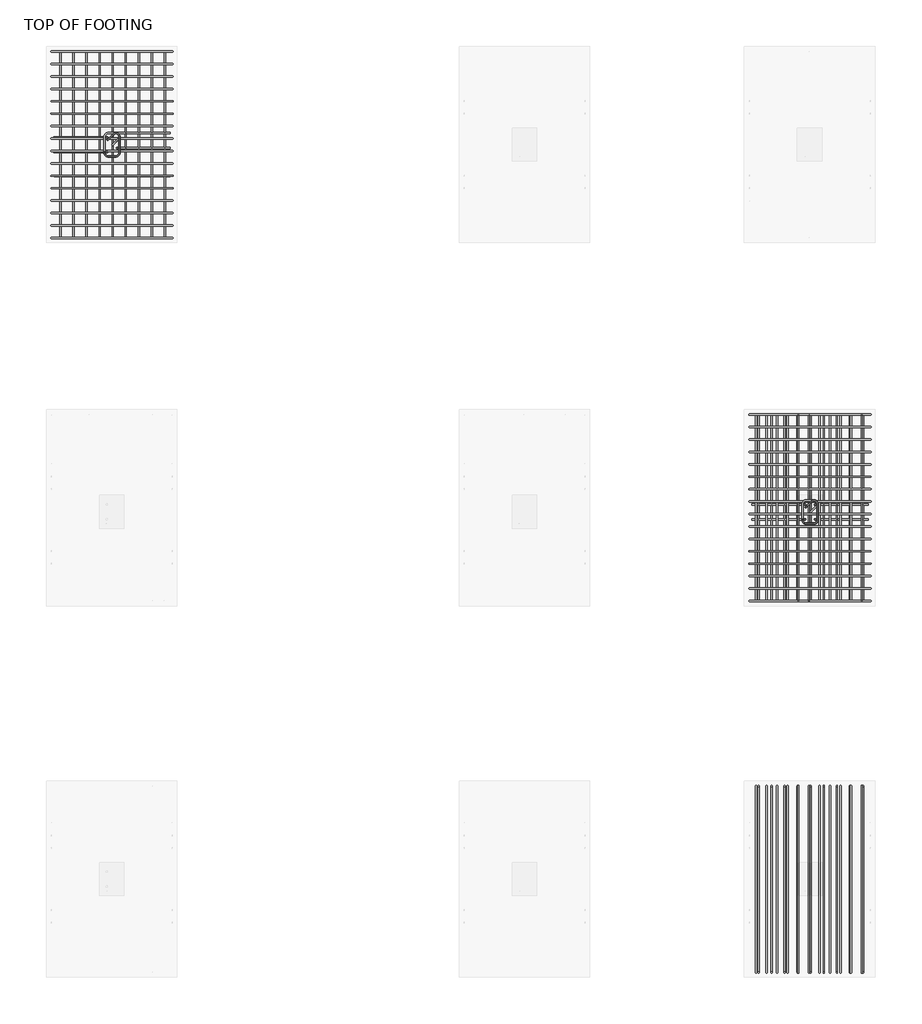
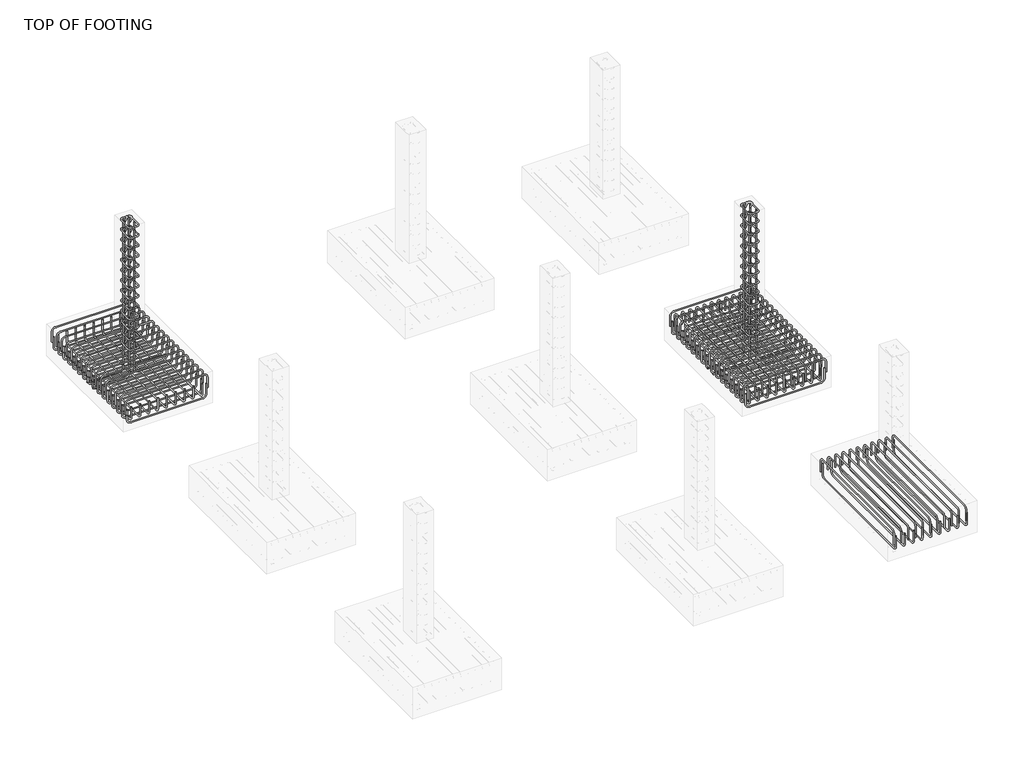
# One storey, part 7 of 8: 15 reinforcing bars.
"""IFC4 building model written with IfcOpenShell, lengths in millimetres."""

from ifc_helpers import new_model, si_unit, point, frame, origin, place, context, project, spatial, polyline, circle_curve, trimmed, segment, composite_curve, source, transform, mapped, element, save
from ifc_brep_helpers import swept_disk

model = new_model("IFC4")

# Units and contexts
model_context = context("Model", 3, world=origin())
ifc_project = project(units=[si_unit("LENGTHUNIT", "METRE", prefix="MILLI")], contexts=[model_context])

# Site, building, storey
site = spatial("IfcSite", under=ifc_project)
building = spatial("IfcBuilding", under=site)
storey = spatial("IfcBuildingStorey", under=building, Name="TOP OF FOOTING", Elevation=-1828.8)

# Reinforcing bars
placement = place(None, origin())
reinforcing_bar_shape = source(origin(), model_context, "Body", "SolidModel", [
    swept_disk(composite_curve([segment(polyline([(3061.4817577, 8966.4007933, -46.35), (3117.2253207, 9022.1443562, -46.35)]), True, "CONTINUOUS"), segment(trimmed(circle_curve(frame((3139.3931183, 8999.9765586, -46.35), z_axis=(0.0, 0.0, -1.0), x_axis=(-22.167797600000085, 22.167797600000995, 0.0)), 31.35), [point((3117.2253207, 9022.1443562, -46.35))], [point((3170.7431183, 8999.9765586, -46.35))], True, "CARTESIAN"), True, "CONTINUOUS"), segment(polyline([(3170.7431183, 8999.9765586, -46.35), (3170.7431183, 8850.5765586, -46.35)]), True, "CONTINUOUS"), segment(trimmed(circle_curve(frame((3139.3931183, 8850.5765586, -46.35), z_axis=(0.0, 0.0, -1.0), x_axis=(31.34999999999991, 0.0, 0.0)), 31.35), [point((3170.7431183, 8850.5765586, -46.35))], [point((3139.3931183, 8819.2265586, -46.35))], True, "CARTESIAN"), True, "CONTINUOUS"), segment(polyline([(3139.3931183, 8819.2265586, -46.35), (3066.1931183, 8819.2265586, -46.35)]), True, "CONTINUOUS"), segment(trimmed(circle_curve(frame((3066.1931183, 8850.5205096, -44.4761991), z_axis=(0.0, 0.05977036468717588, -0.9982121535551258), x_axis=(0.0, -31.29395100000147, -1.873800899999999)), 31.35), [point((3066.1931183, 8819.2265586, -46.35))], [point((3034.8431183, 8850.5205096, -44.4761991))], True, "CARTESIAN"), True, "CONTINUOUS"), segment(polyline([(3034.8431183, 8850.5205096, -44.4761991), (3034.8431183, 9000.0326076, -35.5238009)]), True, "CONTINUOUS"), segment(trimmed(circle_curve(frame((3066.1931183, 9000.0326076, -35.5238009), z_axis=(0.0, 0.05977036468717588, -0.9982121535551258), x_axis=(-31.350000000000364, 0.0, 0.0)), 31.35), [point((3034.8431183, 9000.0326076, -35.5238009))], [point((3066.1931183, 9031.3265586, -33.65))], True, "CARTESIAN"), True, "CONTINUOUS"), segment(polyline([(3066.1931183, 9031.3265586, -33.65), (3139.3931183, 9031.3265586, -33.65)]), True, "CONTINUOUS"), segment(trimmed(circle_curve(frame((3139.3931183, 8999.9765586, -33.65), z_axis=(0.0, 0.0, -1.0), x_axis=(0.0, 31.350000000000364, 0.0)), 31.35), [point((3139.3931183, 9031.3265586, -33.65))], [point((3161.5609159, 8977.808761, -33.65))], True, "CARTESIAN"), True, "CONTINUOUS"), segment(polyline([(3161.5609159, 8977.808761, -33.65), (3105.8173529, 8922.0651981, -33.65)]), True, "CONTINUOUS")], self_intersect=False), 6.35),
])
element("IfcReinforcingBar", 1, at=placement, inside=storey, context=model_context, shape_type="MappedRepresentation", body=[
    mapped(reinforcing_bar_shape, transform((0.0, 0.0, 0.0), x_axis=(1.0, 0.0, 0.0), y_axis=(0.0, 1.0, 0.0), z_axis=(0.0, 0.0, 1.0))),
    mapped(reinforcing_bar_shape, transform((0.0, 0.0, -144.675), x_axis=(1.0, 0.0, 0.0), y_axis=(0.0, 1.0, 0.0), z_axis=(0.0, 0.0, 1.0))),
    mapped(reinforcing_bar_shape, transform((0.0, 0.0, -289.35), x_axis=(1.0, 0.0, 0.0), y_axis=(0.0, 1.0, 0.0), z_axis=(0.0, 0.0, 1.0))),
    mapped(reinforcing_bar_shape, transform((0.0, 0.0, -434.025), x_axis=(1.0, 0.0, 0.0), y_axis=(0.0, 1.0, 0.0), z_axis=(0.0, 0.0, 1.0))),
    mapped(reinforcing_bar_shape, transform((0.0, 0.0, -578.7), x_axis=(1.0, 0.0, 0.0), y_axis=(0.0, 1.0, 0.0), z_axis=(0.0, 0.0, 1.0))),
    mapped(reinforcing_bar_shape, transform((0.0, 0.0, -723.375), x_axis=(1.0, 0.0, 0.0), y_axis=(0.0, 1.0, 0.0), z_axis=(0.0, 0.0, 1.0))),
    mapped(reinforcing_bar_shape, transform((0.0, 0.0, -868.05), x_axis=(1.0, 0.0, 0.0), y_axis=(0.0, 1.0, 0.0), z_axis=(0.0, 0.0, 1.0))),
    mapped(reinforcing_bar_shape, transform((0.0, 0.0, -1012.725), x_axis=(1.0, 0.0, 0.0), y_axis=(0.0, 1.0, 0.0), z_axis=(0.0, 0.0, 1.0))),
    mapped(reinforcing_bar_shape, transform((0.0, 0.0, -1157.4), x_axis=(1.0, 0.0, 0.0), y_axis=(0.0, 1.0, 0.0), z_axis=(0.0, 0.0, 1.0))),
    mapped(reinforcing_bar_shape, transform((0.0, 0.0, -1302.075), x_axis=(1.0, 0.0, 0.0), y_axis=(0.0, 1.0, 0.0), z_axis=(0.0, 0.0, 1.0))),
    mapped(reinforcing_bar_shape, transform((0.0, 0.0, -1446.75), x_axis=(1.0, 0.0, 0.0), y_axis=(0.0, 1.0, 0.0), z_axis=(0.0, 0.0, 1.0))),
    mapped(reinforcing_bar_shape, transform((0.0, 0.0, -1591.425), x_axis=(1.0, 0.0, 0.0), y_axis=(0.0, 1.0, 0.0), z_axis=(0.0, 0.0, 1.0))),
    mapped(reinforcing_bar_shape, transform((0.0, 0.0, -1736.1), x_axis=(1.0, 0.0, 0.0), y_axis=(0.0, 1.0, 0.0), z_axis=(0.0, 0.0, 1.0))),
])
reinforcing_bar_2_shape = source(origin(), model_context, "Body", "SolidModel", [
    swept_disk(composite_curve([segment(polyline([(3635.819602, 8895.4265586, -2177.1384798), (3194.6627797, 8895.4265586, -2177.1384798)]), True, "CONTINUOUS"), segment(trimmed(circle_curve(frame((3194.6627797, 8895.4265586, -2130.7884798), z_axis=(0.0, 1.0, 0.0), x_axis=(0.0, 0.0, -46.34999999999991)), 46.35), [point((3194.6627797, 8895.4265586, -2177.1384798))], [point((3148.3127797, 8895.4265586, -2130.7884798))], True, "CARTESIAN"), True, "CONTINUOUS"), segment(polyline([(3148.3127797, 8895.4265586, -2130.7884798), (3148.3127797, 8895.4265586, -40.0)]), True, "CONTINUOUS")], self_intersect=False), 6.35),
])
element("IfcReinforcingBar", 2, at=placement, inside=storey, context=model_context, shape_type="MappedRepresentation", body=[
    mapped(reinforcing_bar_2_shape, transform((0.0, 0.0, 0.0), x_axis=(1.0, 0.0, 0.0), y_axis=(0.0, 1.0, 0.0), z_axis=(0.0, 0.0, 1.0))),
    mapped(reinforcing_bar_2_shape, transform((0.0, 135.9, 0.0), x_axis=(1.0, 0.0, 0.0), y_axis=(0.0, 1.0, 0.0), z_axis=(0.0, 0.0, 1.0))),
])
reinforcing_bar_3_shape = source(origin(), model_context, "Body", "SolidModel", [
    swept_disk(composite_curve([segment(polyline([(2569.7666346, 8857.3265586, -2177.1384798), (3010.9234568, 8857.3265586, -2177.1384798)]), True, "CONTINUOUS"), segment(trimmed(circle_curve(frame((3010.9234568, 8857.3265586, -2130.7884798), z_axis=(0.0, -1.0, 0.0), x_axis=(0.0, 0.0, -46.34999999999991)), 46.35), [point((3010.9234568, 8857.3265586, -2177.1384798))], [point((3057.2734568, 8857.3265586, -2130.7884798))], True, "CARTESIAN"), True, "CONTINUOUS"), segment(polyline([(3057.2734568, 8857.3265586, -2130.7884798), (3057.2734568, 8857.3265586, -40.0)]), True, "CONTINUOUS")], self_intersect=False), 6.35),
])
element("IfcReinforcingBar", 3, at=placement, inside=storey, context=model_context, shape_type="MappedRepresentation", body=[
    mapped(reinforcing_bar_3_shape, transform((0.0, 0.0, 0.0), x_axis=(1.0, 0.0, 0.0), y_axis=(0.0, 1.0, 0.0), z_axis=(0.0, 0.0, 1.0))),
    mapped(reinforcing_bar_3_shape, transform((0.0, 135.9, 0.0), x_axis=(1.0, 0.0, 0.0), y_axis=(0.0, 1.0, 0.0), z_axis=(0.0, 0.0, 1.0))),
])
reinforcing_bar_4_shape = source(origin(), model_context, "Body", "SolidModel", [
    swept_disk(composite_curve([segment(polyline([(9462.2817577, 5600.7423139, -46.35), (9518.0253207, 5656.4858768, -46.35)]), True, "CONTINUOUS"), segment(trimmed(circle_curve(frame((9540.1931183, 5634.3180792, -46.35), z_axis=(0.0, 0.0, -1.0), x_axis=(-22.167797599999176, 22.167797600000085, 0.0)), 31.35), [point((9518.0253207, 5656.4858768, -46.35))], [point((9571.5431183, 5634.3180792, -46.35))], True, "CARTESIAN"), True, "CONTINUOUS"), segment(polyline([(9571.5431183, 5634.3180792, -46.35), (9571.5431183, 5484.9180792, -46.35)]), True, "CONTINUOUS"), segment(trimmed(circle_curve(frame((9540.1931183, 5484.9180792, -46.35), z_axis=(0.0, 0.0, -1.0), x_axis=(31.350000000000364, 0.0, 0.0)), 31.35), [point((9571.5431183, 5484.9180792, -46.35))], [point((9540.1931183, 5453.5680792, -46.35))], True, "CARTESIAN"), True, "CONTINUOUS"), segment(polyline([(9540.1931183, 5453.5680792, -46.35), (9466.9931183, 5453.5680792, -46.35)]), True, "CONTINUOUS"), segment(trimmed(circle_curve(frame((9466.9931183, 5484.8620303, -44.4761991), z_axis=(0.0, 0.05977036468717588, -0.9982121535551258), x_axis=(0.0, -31.293951099999504, -1.873800899999999)), 31.35), [point((9466.9931183, 5453.5680792, -46.35))], [point((9435.6431183, 5484.8620303, -44.4761991))], True, "CARTESIAN"), True, "CONTINUOUS"), segment(polyline([(9435.6431183, 5484.8620303, -44.4761991), (9435.6431183, 5634.3741282, -35.5238009)]), True, "CONTINUOUS"), segment(trimmed(circle_curve(frame((9466.9931183, 5634.3741282, -35.5238009), z_axis=(0.0, 0.05977036468717588, -0.9982121535551258), x_axis=(-31.350000000000364, 0.0, 0.0)), 31.35), [point((9435.6431183, 5634.3741282, -35.5238009))], [point((9466.9931183, 5665.6680792, -33.65))], True, "CARTESIAN"), True, "CONTINUOUS"), segment(polyline([(9466.9931183, 5665.6680792, -33.65), (9540.1931183, 5665.6680792, -33.65)]), True, "CONTINUOUS"), segment(trimmed(circle_curve(frame((9540.1931183, 5634.3180792, -33.65), z_axis=(0.0, 0.0, -1.0), x_axis=(0.0, 31.349999999999454, 0.0)), 31.35), [point((9540.1931183, 5665.6680792, -33.65))], [point((9562.3609159, 5612.1502816, -33.65))], True, "CARTESIAN"), True, "CONTINUOUS"), segment(polyline([(9562.3609159, 5612.1502816, -33.65), (9506.6173529, 5556.4067187, -33.65)]), True, "CONTINUOUS")], self_intersect=False), 6.35),
])
element("IfcReinforcingBar", 4, at=placement, inside=storey, context=model_context, shape_type="MappedRepresentation", body=[
    mapped(reinforcing_bar_4_shape, transform((0.0, 0.0, 0.0), x_axis=(1.0, 0.0, 0.0), y_axis=(0.0, 1.0, 0.0), z_axis=(0.0, 0.0, 1.0))),
    mapped(reinforcing_bar_4_shape, transform((0.0, 0.0, -144.675), x_axis=(1.0, 0.0, 0.0), y_axis=(0.0, 1.0, 0.0), z_axis=(0.0, 0.0, 1.0))),
    mapped(reinforcing_bar_4_shape, transform((0.0, 0.0, -289.35), x_axis=(1.0, 0.0, 0.0), y_axis=(0.0, 1.0, 0.0), z_axis=(0.0, 0.0, 1.0))),
    mapped(reinforcing_bar_4_shape, transform((0.0, 0.0, -434.025), x_axis=(1.0, 0.0, 0.0), y_axis=(0.0, 1.0, 0.0), z_axis=(0.0, 0.0, 1.0))),
    mapped(reinforcing_bar_4_shape, transform((0.0, 0.0, -578.7), x_axis=(1.0, 0.0, 0.0), y_axis=(0.0, 1.0, 0.0), z_axis=(0.0, 0.0, 1.0))),
    mapped(reinforcing_bar_4_shape, transform((0.0, 0.0, -723.375), x_axis=(1.0, 0.0, 0.0), y_axis=(0.0, 1.0, 0.0), z_axis=(0.0, 0.0, 1.0))),
    mapped(reinforcing_bar_4_shape, transform((0.0, 0.0, -868.05), x_axis=(1.0, 0.0, 0.0), y_axis=(0.0, 1.0, 0.0), z_axis=(0.0, 0.0, 1.0))),
    mapped(reinforcing_bar_4_shape, transform((0.0, 0.0, -1012.725), x_axis=(1.0, 0.0, 0.0), y_axis=(0.0, 1.0, 0.0), z_axis=(0.0, 0.0, 1.0))),
    mapped(reinforcing_bar_4_shape, transform((0.0, 0.0, -1157.4), x_axis=(1.0, 0.0, 0.0), y_axis=(0.0, 1.0, 0.0), z_axis=(0.0, 0.0, 1.0))),
    mapped(reinforcing_bar_4_shape, transform((0.0, 0.0, -1302.075), x_axis=(1.0, 0.0, 0.0), y_axis=(0.0, 1.0, 0.0), z_axis=(0.0, 0.0, 1.0))),
    mapped(reinforcing_bar_4_shape, transform((0.0, 0.0, -1446.75), x_axis=(1.0, 0.0, 0.0), y_axis=(0.0, 1.0, 0.0), z_axis=(0.0, 0.0, 1.0))),
    mapped(reinforcing_bar_4_shape, transform((0.0, 0.0, -1591.425), x_axis=(1.0, 0.0, 0.0), y_axis=(0.0, 1.0, 0.0), z_axis=(0.0, 0.0, 1.0))),
    mapped(reinforcing_bar_4_shape, transform((0.0, 0.0, -1736.1), x_axis=(1.0, 0.0, 0.0), y_axis=(0.0, 1.0, 0.0), z_axis=(0.0, 0.0, 1.0))),
])
reinforcing_bar_5_shape = source(origin(), model_context, "Body", "SolidModel", [
    swept_disk(composite_curve([segment(polyline([(10036.619602, 5491.6680792, -2177.1384798), (9595.4627797, 5491.6680792, -2177.1384798)]), True, "CONTINUOUS"), segment(trimmed(circle_curve(frame((9595.4627797, 5491.6680792, -2130.7884798), z_axis=(0.0, 1.0, 0.0), x_axis=(0.0, 0.0, -46.34999999999991)), 46.35), [point((9595.4627797, 5491.6680792, -2177.1384798))], [point((9549.1127797, 5491.6680792, -2130.7884798))], True, "CARTESIAN"), True, "CONTINUOUS"), segment(polyline([(9549.1127797, 5491.6680792, -2130.7884798), (9549.1127797, 5491.6680792, -40.0)]), True, "CONTINUOUS")], self_intersect=False), 6.35),
])
element("IfcReinforcingBar", 5, at=placement, inside=storey, context=model_context, shape_type="MappedRepresentation", body=[
    mapped(reinforcing_bar_5_shape, transform((0.0, 0.0, 0.0), x_axis=(1.0, 0.0, 0.0), y_axis=(0.0, 1.0, 0.0), z_axis=(0.0, 0.0, 1.0))),
    mapped(reinforcing_bar_5_shape, transform((0.0, 135.9, 0.0), x_axis=(1.0, 0.0, 0.0), y_axis=(0.0, 1.0, 0.0), z_axis=(0.0, 0.0, 1.0))),
])
reinforcing_bar_6_shape = source(origin(), model_context, "Body", "SolidModel", [
    swept_disk(composite_curve([segment(polyline([(8970.5666346, 5491.6680792, -2177.1384798), (9411.7234568, 5491.6680792, -2177.1384798)]), True, "CONTINUOUS"), segment(trimmed(circle_curve(frame((9411.7234568, 5491.6680792, -2130.7884798), z_axis=(0.0, -1.0, 0.0), x_axis=(0.0, 0.0, -46.34999999999991)), 46.35), [point((9411.7234568, 5491.6680792, -2177.1384798))], [point((9458.0734568, 5491.6680792, -2130.7884798))], True, "CARTESIAN"), True, "CONTINUOUS"), segment(polyline([(9458.0734568, 5491.6680792, -2130.7884798), (9458.0734568, 5491.6680792, -40.0)]), True, "CONTINUOUS")], self_intersect=False), 6.35),
])
element("IfcReinforcingBar", 6, at=placement, inside=storey, context=model_context, shape_type="MappedRepresentation", body=[
    mapped(reinforcing_bar_6_shape, transform((0.0, 0.0, 0.0), x_axis=(1.0, 0.0, 0.0), y_axis=(0.0, 1.0, 0.0), z_axis=(0.0, 0.0, 1.0))),
    mapped(reinforcing_bar_6_shape, transform((0.0, 135.9, 0.0), x_axis=(1.0, 0.0, 0.0), y_axis=(0.0, 1.0, 0.0), z_axis=(0.0, 0.0, 1.0))),
])
reinforcing_bar_7_shape = source(origin(), model_context, "Body", "SolidModel", [
    swept_disk(composite_curve([segment(polyline([(3637.0426771, 9778.9265586, -2008.2544267), (3637.0426771, 9778.9265586, -2155.5544267)]), True, "CONTINUOUS"), segment(trimmed(circle_curve(frame((3590.6926771, 9778.9265586, -2155.5544267), z_axis=(0.0, 1.0, 0.0), x_axis=(46.350000000000364, 0.0, 0.0)), 46.35), [point((3637.0426771, 9778.9265586, -2155.5544267))], [point((3590.6926771, 9778.9265586, -2201.9044267))], True, "CARTESIAN"), True, "CONTINUOUS"), segment(polyline([(3590.6926771, 9778.9265586, -2201.9044267), (2619.6766408, 9778.9265586, -2201.9044267)]), True, "CONTINUOUS"), segment(trimmed(circle_curve(frame((2619.6766408, 9778.9265586, -2155.5544267), z_axis=(0.0, 1.0, 0.0), x_axis=(0.0, 0.0, -46.34999999999991)), 46.35), [point((2619.6766408, 9778.9265586, -2201.9044267))], [point((2573.3266408, 9778.9265586, -2155.5544267))], True, "CARTESIAN"), True, "CONTINUOUS"), segment(polyline([(2573.3266408, 9778.9265586, -2155.5544267), (2573.3266408, 9778.9265586, -2008.2544267)]), True, "CONTINUOUS")], self_intersect=False), 6.35),
])
element("IfcReinforcingBar", 7, at=placement, inside=storey, context=model_context, shape_type="MappedRepresentation", body=[
    mapped(reinforcing_bar_7_shape, transform((0.0, 0.0, 0.0), x_axis=(1.0, 0.0, 0.0), y_axis=(0.0, 1.0, 0.0), z_axis=(0.0, 0.0, 1.0))),
    mapped(reinforcing_bar_7_shape, transform((0.0, -113.82, 0.0), x_axis=(1.0, 0.0, 0.0), y_axis=(0.0, 1.0, 0.0), z_axis=(0.0, 0.0, 1.0))),
    mapped(reinforcing_bar_7_shape, transform((0.0, -227.64, 0.0), x_axis=(1.0, 0.0, 0.0), y_axis=(0.0, 1.0, 0.0), z_axis=(0.0, 0.0, 1.0))),
    mapped(reinforcing_bar_7_shape, transform((0.0, -341.46, 0.0), x_axis=(1.0, 0.0, 0.0), y_axis=(0.0, 1.0, 0.0), z_axis=(0.0, 0.0, 1.0))),
    mapped(reinforcing_bar_7_shape, transform((0.0, -455.28, 0.0), x_axis=(1.0, 0.0, 0.0), y_axis=(0.0, 1.0, 0.0), z_axis=(0.0, 0.0, 1.0))),
    mapped(reinforcing_bar_7_shape, transform((0.0, -569.1, 0.0), x_axis=(1.0, 0.0, 0.0), y_axis=(0.0, 1.0, 0.0), z_axis=(0.0, 0.0, 1.0))),
    mapped(reinforcing_bar_7_shape, transform((0.0, -682.92, 0.0), x_axis=(1.0, 0.0, 0.0), y_axis=(0.0, 1.0, 0.0), z_axis=(0.0, 0.0, 1.0))),
    mapped(reinforcing_bar_7_shape, transform((0.0, -796.74, 0.0), x_axis=(1.0, 0.0, 0.0), y_axis=(0.0, 1.0, 0.0), z_axis=(0.0, 0.0, 1.0))),
    mapped(reinforcing_bar_7_shape, transform((0.0, -910.56, 0.0), x_axis=(1.0, 0.0, 0.0), y_axis=(0.0, 1.0, 0.0), z_axis=(0.0, 0.0, 1.0))),
    mapped(reinforcing_bar_7_shape, transform((0.0, -1024.38, 0.0), x_axis=(1.0, 0.0, 0.0), y_axis=(0.0, 1.0, 0.0), z_axis=(0.0, 0.0, 1.0))),
    mapped(reinforcing_bar_7_shape, transform((0.0, -1138.2, 0.0), x_axis=(1.0, 0.0, 0.0), y_axis=(0.0, 1.0, 0.0), z_axis=(0.0, 0.0, 1.0))),
    mapped(reinforcing_bar_7_shape, transform((0.0, -1252.02, 0.0), x_axis=(1.0, 0.0, 0.0), y_axis=(0.0, 1.0, 0.0), z_axis=(0.0, 0.0, 1.0))),
    mapped(reinforcing_bar_7_shape, transform((0.0, -1365.84, 0.0), x_axis=(1.0, 0.0, 0.0), y_axis=(0.0, 1.0, 0.0), z_axis=(0.0, 0.0, 1.0))),
    mapped(reinforcing_bar_7_shape, transform((0.0, -1479.66, 0.0), x_axis=(1.0, 0.0, 0.0), y_axis=(0.0, 1.0, 0.0), z_axis=(0.0, 0.0, 1.0))),
    mapped(reinforcing_bar_7_shape, transform((0.0, -1593.48, 0.0), x_axis=(1.0, 0.0, 0.0), y_axis=(0.0, 1.0, 0.0), z_axis=(0.0, 0.0, 1.0))),
    mapped(reinforcing_bar_7_shape, transform((0.0, -1707.3, 0.0), x_axis=(1.0, 0.0, 0.0), y_axis=(0.0, 1.0, 0.0), z_axis=(0.0, 0.0, 1.0))),
])
reinforcing_bar_8_shape = source(origin(), model_context, "Body", "SolidModel", [
    swept_disk(composite_curve([segment(polyline([(2549.1431183, 9778.9265586, -2068.8), (2549.1431183, 9778.9265586, -1921.5)]), True, "CONTINUOUS"), segment(trimmed(circle_curve(frame((2595.4931183, 9778.9265586, -1921.5), z_axis=(0.0, 1.0, 0.0), x_axis=(-46.34999999999991, 0.0, 0.0)), 46.35), [point((2549.1431183, 9778.9265586, -1921.5))], [point((2595.4931183, 9778.9265586, -1875.15))], True, "CARTESIAN"), True, "CONTINUOUS"), segment(polyline([(2595.4931183, 9778.9265586, -1875.15), (3610.0931183, 9778.9265586, -1875.15)]), True, "CONTINUOUS"), segment(trimmed(circle_curve(frame((3610.0931183, 9778.9265586, -1921.5), z_axis=(0.0, 1.0, 0.0), x_axis=(0.0, 0.0, 46.34999999999991)), 46.35), [point((3610.0931183, 9778.9265586, -1875.15))], [point((3656.4431183, 9778.9265586, -1921.5))], True, "CARTESIAN"), True, "CONTINUOUS"), segment(polyline([(3656.4431183, 9778.9265586, -1921.5), (3656.4431183, 9778.9265586, -2068.8)]), True, "CONTINUOUS")], self_intersect=False), 6.35),
])
element("IfcReinforcingBar", 8, at=placement, inside=storey, context=model_context, shape_type="MappedRepresentation", body=[
    mapped(reinforcing_bar_8_shape, transform((0.0, 0.0, 0.0), x_axis=(1.0, 0.0, 0.0), y_axis=(0.0, 1.0, 0.0), z_axis=(0.0, 0.0, 1.0))),
    mapped(reinforcing_bar_8_shape, transform((0.0, -113.82, 0.0), x_axis=(1.0, 0.0, 0.0), y_axis=(0.0, 1.0, 0.0), z_axis=(0.0, 0.0, 1.0))),
    mapped(reinforcing_bar_8_shape, transform((0.0, -227.64, 0.0), x_axis=(1.0, 0.0, 0.0), y_axis=(0.0, 1.0, 0.0), z_axis=(0.0, 0.0, 1.0))),
    mapped(reinforcing_bar_8_shape, transform((0.0, -341.46, 0.0), x_axis=(1.0, 0.0, 0.0), y_axis=(0.0, 1.0, 0.0), z_axis=(0.0, 0.0, 1.0))),
    mapped(reinforcing_bar_8_shape, transform((0.0, -455.28, 0.0), x_axis=(1.0, 0.0, 0.0), y_axis=(0.0, 1.0, 0.0), z_axis=(0.0, 0.0, 1.0))),
    mapped(reinforcing_bar_8_shape, transform((0.0, -569.1, 0.0), x_axis=(1.0, 0.0, 0.0), y_axis=(0.0, 1.0, 0.0), z_axis=(0.0, 0.0, 1.0))),
    mapped(reinforcing_bar_8_shape, transform((0.0, -682.92, 0.0), x_axis=(1.0, 0.0, 0.0), y_axis=(0.0, 1.0, 0.0), z_axis=(0.0, 0.0, 1.0))),
    mapped(reinforcing_bar_8_shape, transform((0.0, -796.74, 0.0), x_axis=(1.0, 0.0, 0.0), y_axis=(0.0, 1.0, 0.0), z_axis=(0.0, 0.0, 1.0))),
    mapped(reinforcing_bar_8_shape, transform((0.0, -910.56, 0.0), x_axis=(1.0, 0.0, 0.0), y_axis=(0.0, 1.0, 0.0), z_axis=(0.0, 0.0, 1.0))),
    mapped(reinforcing_bar_8_shape, transform((0.0, -1024.38, 0.0), x_axis=(1.0, 0.0, 0.0), y_axis=(0.0, 1.0, 0.0), z_axis=(0.0, 0.0, 1.0))),
    mapped(reinforcing_bar_8_shape, transform((0.0, -1138.2, 0.0), x_axis=(1.0, 0.0, 0.0), y_axis=(0.0, 1.0, 0.0), z_axis=(0.0, 0.0, 1.0))),
    mapped(reinforcing_bar_8_shape, transform((0.0, -1252.02, 0.0), x_axis=(1.0, 0.0, 0.0), y_axis=(0.0, 1.0, 0.0), z_axis=(0.0, 0.0, 1.0))),
    mapped(reinforcing_bar_8_shape, transform((0.0, -1365.84, 0.0), x_axis=(1.0, 0.0, 0.0), y_axis=(0.0, 1.0, 0.0), z_axis=(0.0, 0.0, 1.0))),
    mapped(reinforcing_bar_8_shape, transform((0.0, -1479.66, 0.0), x_axis=(1.0, 0.0, 0.0), y_axis=(0.0, 1.0, 0.0), z_axis=(0.0, 0.0, 1.0))),
    mapped(reinforcing_bar_8_shape, transform((0.0, -1593.48, 0.0), x_axis=(1.0, 0.0, 0.0), y_axis=(0.0, 1.0, 0.0), z_axis=(0.0, 0.0, 1.0))),
    mapped(reinforcing_bar_8_shape, transform((0.0, -1707.3, 0.0), x_axis=(1.0, 0.0, 0.0), y_axis=(0.0, 1.0, 0.0), z_axis=(0.0, 0.0, 1.0))),
])
reinforcing_bar_9_shape = source(origin(), model_context, "Body", "SolidModel", [
    swept_disk(composite_curve([segment(polyline([(2631.3651697, 9778.9265586, -1986.9111268), (2631.3651697, 9778.9265586, -2134.2111268)]), True, "CONTINUOUS"), segment(trimmed(circle_curve(frame((2631.3651697, 9732.5765586, -2134.2111268), z_axis=(-1.0, 0.0, 0.0), x_axis=(0.0, 46.350000000000364, 0.0)), 46.35), [point((2631.3651697, 9778.9265586, -2134.2111268))], [point((2631.3651697, 9732.5765586, -2180.5611268))], True, "CARTESIAN"), True, "CONTINUOUS"), segment(polyline([(2631.3651697, 9732.5765586, -2180.5611268), (2631.3651697, 8117.9765586, -2180.5611268)]), True, "CONTINUOUS"), segment(trimmed(circle_curve(frame((2631.3651697, 8117.9765586, -2134.2111268), z_axis=(-1.0, 0.0, 0.0), x_axis=(0.0, 0.0, -46.34999999999991)), 46.35), [point((2631.3651697, 8117.9765586, -2180.5611268))], [point((2631.3651697, 8071.6265586, -2134.2111268))], True, "CARTESIAN"), True, "CONTINUOUS"), segment(polyline([(2631.3651697, 8071.6265586, -2134.2111268), (2631.3651697, 8071.6265586, -1986.9111268)]), True, "CONTINUOUS")], self_intersect=False), 6.35),
])
element("IfcReinforcingBar", 9, at=placement, inside=storey, context=model_context, shape_type="MappedRepresentation", body=[
    mapped(reinforcing_bar_9_shape, transform((0.0, 0.0, 0.0), x_axis=(1.0, 0.0, 0.0), y_axis=(0.0, 1.0, 0.0), z_axis=(0.0, 0.0, 1.0))),
    mapped(reinforcing_bar_9_shape, transform((119.5564677, 0.0, 0.0), x_axis=(1.0, 0.0, 0.0), y_axis=(0.0, 1.0, 0.0), z_axis=(0.0, 0.0, 1.0))),
    mapped(reinforcing_bar_9_shape, transform((239.1129355, 0.0, 0.0), x_axis=(1.0, 0.0, 0.0), y_axis=(0.0, 1.0, 0.0), z_axis=(0.0, 0.0, 1.0))),
    mapped(reinforcing_bar_9_shape, transform((358.6694032, 0.0, 0.0), x_axis=(1.0, 0.0, 0.0), y_axis=(0.0, 1.0, 0.0), z_axis=(0.0, 0.0, 1.0))),
    mapped(reinforcing_bar_9_shape, transform((478.2258709, 0.0, 0.0), x_axis=(1.0, 0.0, 0.0), y_axis=(0.0, 1.0, 0.0), z_axis=(0.0, 0.0, 1.0))),
    mapped(reinforcing_bar_9_shape, transform((597.7823387, 0.0, 0.0), x_axis=(1.0, 0.0, 0.0), y_axis=(0.0, 1.0, 0.0), z_axis=(0.0, 0.0, 1.0))),
    mapped(reinforcing_bar_9_shape, transform((717.3388064, 0.0, 0.0), x_axis=(1.0, 0.0, 0.0), y_axis=(0.0, 1.0, 0.0), z_axis=(0.0, 0.0, 1.0))),
    mapped(reinforcing_bar_9_shape, transform((836.8952741, 0.0, 0.0), x_axis=(1.0, 0.0, 0.0), y_axis=(0.0, 1.0, 0.0), z_axis=(0.0, 0.0, 1.0))),
    mapped(reinforcing_bar_9_shape, transform((956.4517419, 0.0, 0.0), x_axis=(1.0, 0.0, 0.0), y_axis=(0.0, 1.0, 0.0), z_axis=(0.0, 0.0, 1.0))),
])
reinforcing_bar_10_shape = source(origin(), model_context, "Body", "SolidModel", [
    swept_disk(composite_curve([segment(polyline([(9032.1651697, 3047.9265586, -1986.9111268), (9032.1651697, 3047.9265586, -2134.2111268)]), True, "CONTINUOUS"), segment(trimmed(circle_curve(frame((9032.1651697, 3001.5765586, -2134.2111268), z_axis=(-1.0, 0.0, 0.0), x_axis=(0.0, 46.34999999999991, 0.0)), 46.35), [point((9032.1651697, 3047.9265586, -2134.2111268))], [point((9032.1651697, 3001.5765586, -2180.5611268))], True, "CARTESIAN"), True, "CONTINUOUS"), segment(polyline([(9032.1651697, 3001.5765586, -2180.5611268), (9032.1651697, 1386.9765586, -2180.5611268)]), True, "CONTINUOUS"), segment(trimmed(circle_curve(frame((9032.1651697, 1386.9765586, -2134.2111268), z_axis=(-1.0, 0.0, 0.0), x_axis=(0.0, 0.0, -46.34999999999991)), 46.35), [point((9032.1651697, 1386.9765586, -2180.5611268))], [point((9032.1651697, 1340.6265586, -2134.2111268))], True, "CARTESIAN"), True, "CONTINUOUS"), segment(polyline([(9032.1651697, 1340.6265586, -2134.2111268), (9032.1651697, 1340.6265586, -1986.9111268)]), True, "CONTINUOUS")], self_intersect=False), 6.35),
])
element("IfcReinforcingBar", 10, at=placement, inside=storey, context=model_context, shape_type="MappedRepresentation", body=[
    mapped(reinforcing_bar_10_shape, transform((0.0, 0.0, 0.0), x_axis=(1.0, 0.0, 0.0), y_axis=(0.0, 1.0, 0.0), z_axis=(0.0, 0.0, 1.0))),
    mapped(reinforcing_bar_10_shape, transform((119.5564677, 0.0, 0.0), x_axis=(1.0, 0.0, 0.0), y_axis=(0.0, 1.0, 0.0), z_axis=(0.0, 0.0, 1.0))),
    mapped(reinforcing_bar_10_shape, transform((239.1129355, 0.0, 0.0), x_axis=(1.0, 0.0, 0.0), y_axis=(0.0, 1.0, 0.0), z_axis=(0.0, 0.0, 1.0))),
    mapped(reinforcing_bar_10_shape, transform((358.6694032, 0.0, 0.0), x_axis=(1.0, 0.0, 0.0), y_axis=(0.0, 1.0, 0.0), z_axis=(0.0, 0.0, 1.0))),
    mapped(reinforcing_bar_10_shape, transform((478.2258709, 0.0, 0.0), x_axis=(1.0, 0.0, 0.0), y_axis=(0.0, 1.0, 0.0), z_axis=(0.0, 0.0, 1.0))),
    mapped(reinforcing_bar_10_shape, transform((597.7823387, 0.0, 0.0), x_axis=(1.0, 0.0, 0.0), y_axis=(0.0, 1.0, 0.0), z_axis=(0.0, 0.0, 1.0))),
    mapped(reinforcing_bar_10_shape, transform((717.3388064, 0.0, 0.0), x_axis=(1.0, 0.0, 0.0), y_axis=(0.0, 1.0, 0.0), z_axis=(0.0, 0.0, 1.0))),
    mapped(reinforcing_bar_10_shape, transform((836.8952741, 0.0, 0.0), x_axis=(1.0, 0.0, 0.0), y_axis=(0.0, 1.0, 0.0), z_axis=(0.0, 0.0, 1.0))),
    mapped(reinforcing_bar_10_shape, transform((956.4517419, 0.0, 0.0), x_axis=(1.0, 0.0, 0.0), y_axis=(0.0, 1.0, 0.0), z_axis=(0.0, 0.0, 1.0))),
])
reinforcing_bar_11_shape = source(origin(), model_context, "Body", "SolidModel", [
    swept_disk(composite_curve([segment(polyline([(9977.9331701, 3047.9265586, -2094.8977257), (9977.9331701, 3047.9265586, -1947.5977257)]), True, "CONTINUOUS"), segment(trimmed(circle_curve(frame((9977.9331701, 3001.5765586, -1947.5977257), z_axis=(1.0, 0.0, 0.0), x_axis=(0.0, 46.34999999999991, 0.0)), 46.35), [point((9977.9331701, 3047.9265586, -1947.5977257))], [point((9977.9331701, 3001.5765586, -1901.2477257))], True, "CARTESIAN"), True, "CONTINUOUS"), segment(polyline([(9977.9331701, 3001.5765586, -1901.2477257), (9977.9331701, 1386.9765586, -1901.2477257)]), True, "CONTINUOUS"), segment(trimmed(circle_curve(frame((9977.9331701, 1386.9765586, -1947.5977257), z_axis=(1.0, 0.0, 0.0), x_axis=(0.0, 0.0, 46.34999999999991)), 46.35), [point((9977.9331701, 1386.9765586, -1901.2477257))], [point((9977.9331701, 1340.6265586, -1947.5977257))], True, "CARTESIAN"), True, "CONTINUOUS"), segment(polyline([(9977.9331701, 1340.6265586, -1947.5977257), (9977.9331701, 1340.6265586, -2094.8977257)]), True, "CONTINUOUS")], self_intersect=False), 6.35),
])
element("IfcReinforcingBar", 11, at=placement, inside=storey, context=model_context, shape_type="MappedRepresentation", body=[
    mapped(reinforcing_bar_11_shape, transform((0.0, 0.0, 0.0), x_axis=(1.0, 0.0, 0.0), y_axis=(0.0, 1.0, 0.0), z_axis=(0.0, 0.0, 1.0))),
    mapped(reinforcing_bar_11_shape, transform((-97.0050815, 0.0, 0.0), x_axis=(1.0, 0.0, 0.0), y_axis=(0.0, 1.0, 0.0), z_axis=(0.0, 0.0, 1.0))),
    mapped(reinforcing_bar_11_shape, transform((-194.0101631, 0.0, 0.0), x_axis=(1.0, 0.0, 0.0), y_axis=(0.0, 1.0, 0.0), z_axis=(0.0, 0.0, 1.0))),
    mapped(reinforcing_bar_11_shape, transform((-291.0152446, 0.0, 0.0), x_axis=(1.0, 0.0, 0.0), y_axis=(0.0, 1.0, 0.0), z_axis=(0.0, 0.0, 1.0))),
    mapped(reinforcing_bar_11_shape, transform((-388.0203261, 0.0, 0.0), x_axis=(1.0, 0.0, 0.0), y_axis=(0.0, 1.0, 0.0), z_axis=(0.0, 0.0, 1.0))),
    mapped(reinforcing_bar_11_shape, transform((-485.0254076, 0.0, 0.0), x_axis=(1.0, 0.0, 0.0), y_axis=(0.0, 1.0, 0.0), z_axis=(0.0, 0.0, 1.0))),
    mapped(reinforcing_bar_11_shape, transform((-582.0304892, 0.0, 0.0), x_axis=(1.0, 0.0, 0.0), y_axis=(0.0, 1.0, 0.0), z_axis=(0.0, 0.0, 1.0))),
    mapped(reinforcing_bar_11_shape, transform((-679.0355707, 0.0, 0.0), x_axis=(1.0, 0.0, 0.0), y_axis=(0.0, 1.0, 0.0), z_axis=(0.0, 0.0, 1.0))),
    mapped(reinforcing_bar_11_shape, transform((-776.0406522, 0.0, 0.0), x_axis=(1.0, 0.0, 0.0), y_axis=(0.0, 1.0, 0.0), z_axis=(0.0, 0.0, 1.0))),
    mapped(reinforcing_bar_11_shape, transform((-873.0457338, 0.0, 0.0), x_axis=(1.0, 0.0, 0.0), y_axis=(0.0, 1.0, 0.0), z_axis=(0.0, 0.0, 1.0))),
    mapped(reinforcing_bar_11_shape, transform((-970.0508153, 0.0, 0.0), x_axis=(1.0, 0.0, 0.0), y_axis=(0.0, 1.0, 0.0), z_axis=(0.0, 0.0, 1.0))),
])
reinforcing_bar_12_shape = source(origin(), model_context, "Body", "SolidModel", [
    swept_disk(composite_curve([segment(polyline([(10037.8426771, 6451.7662126, -2008.2544267), (10037.8426771, 6451.7662126, -2155.5544267)]), True, "CONTINUOUS"), segment(trimmed(circle_curve(frame((9991.4926771, 6451.7662126, -2155.5544267), z_axis=(0.0, 1.0, 0.0), x_axis=(46.350000000000364, 0.0, 0.0)), 46.35), [point((10037.8426771, 6451.7662126, -2155.5544267))], [point((9991.4926771, 6451.7662126, -2201.9044267))], True, "CARTESIAN"), True, "CONTINUOUS"), segment(polyline([(9991.4926771, 6451.7662126, -2201.9044267), (9020.4766408, 6451.7662126, -2201.9044267)]), True, "CONTINUOUS"), segment(trimmed(circle_curve(frame((9020.4766408, 6451.7662126, -2155.5544267), z_axis=(0.0, 1.0, 0.0), x_axis=(0.0, 0.0, -46.34999999999991)), 46.35), [point((9020.4766408, 6451.7662126, -2201.9044267))], [point((8974.1266408, 6451.7662126, -2155.5544267))], True, "CARTESIAN"), True, "CONTINUOUS"), segment(polyline([(8974.1266408, 6451.7662126, -2155.5544267), (8974.1266408, 6451.7662126, -2008.2544267)]), True, "CONTINUOUS")], self_intersect=False), 6.35),
])
element("IfcReinforcingBar", 12, at=placement, inside=storey, context=model_context, shape_type="MappedRepresentation", body=[
    mapped(reinforcing_bar_12_shape, transform((0.0, 0.0, 0.0), x_axis=(1.0, 0.0, 0.0), y_axis=(0.0, 1.0, 0.0), z_axis=(0.0, 0.0, 1.0))),
    mapped(reinforcing_bar_12_shape, transform((0.0, -113.82, 0.0), x_axis=(1.0, 0.0, 0.0), y_axis=(0.0, 1.0, 0.0), z_axis=(0.0, 0.0, 1.0))),
    mapped(reinforcing_bar_12_shape, transform((0.0, -227.64, 0.0), x_axis=(1.0, 0.0, 0.0), y_axis=(0.0, 1.0, 0.0), z_axis=(0.0, 0.0, 1.0))),
    mapped(reinforcing_bar_12_shape, transform((0.0, -341.46, 0.0), x_axis=(1.0, 0.0, 0.0), y_axis=(0.0, 1.0, 0.0), z_axis=(0.0, 0.0, 1.0))),
    mapped(reinforcing_bar_12_shape, transform((0.0, -455.28, 0.0), x_axis=(1.0, 0.0, 0.0), y_axis=(0.0, 1.0, 0.0), z_axis=(0.0, 0.0, 1.0))),
    mapped(reinforcing_bar_12_shape, transform((0.0, -569.1, 0.0), x_axis=(1.0, 0.0, 0.0), y_axis=(0.0, 1.0, 0.0), z_axis=(0.0, 0.0, 1.0))),
    mapped(reinforcing_bar_12_shape, transform((0.0, -682.92, 0.0), x_axis=(1.0, 0.0, 0.0), y_axis=(0.0, 1.0, 0.0), z_axis=(0.0, 0.0, 1.0))),
    mapped(reinforcing_bar_12_shape, transform((0.0, -796.74, 0.0), x_axis=(1.0, 0.0, 0.0), y_axis=(0.0, 1.0, 0.0), z_axis=(0.0, 0.0, 1.0))),
    mapped(reinforcing_bar_12_shape, transform((0.0, -910.56, 0.0), x_axis=(1.0, 0.0, 0.0), y_axis=(0.0, 1.0, 0.0), z_axis=(0.0, 0.0, 1.0))),
    mapped(reinforcing_bar_12_shape, transform((0.0, -1024.38, 0.0), x_axis=(1.0, 0.0, 0.0), y_axis=(0.0, 1.0, 0.0), z_axis=(0.0, 0.0, 1.0))),
    mapped(reinforcing_bar_12_shape, transform((0.0, -1138.2, 0.0), x_axis=(1.0, 0.0, 0.0), y_axis=(0.0, 1.0, 0.0), z_axis=(0.0, 0.0, 1.0))),
    mapped(reinforcing_bar_12_shape, transform((0.0, -1252.02, 0.0), x_axis=(1.0, 0.0, 0.0), y_axis=(0.0, 1.0, 0.0), z_axis=(0.0, 0.0, 1.0))),
    mapped(reinforcing_bar_12_shape, transform((0.0, -1365.84, 0.0), x_axis=(1.0, 0.0, 0.0), y_axis=(0.0, 1.0, 0.0), z_axis=(0.0, 0.0, 1.0))),
    mapped(reinforcing_bar_12_shape, transform((0.0, -1479.66, 0.0), x_axis=(1.0, 0.0, 0.0), y_axis=(0.0, 1.0, 0.0), z_axis=(0.0, 0.0, 1.0))),
    mapped(reinforcing_bar_12_shape, transform((0.0, -1593.48, 0.0), x_axis=(1.0, 0.0, 0.0), y_axis=(0.0, 1.0, 0.0), z_axis=(0.0, 0.0, 1.0))),
    mapped(reinforcing_bar_12_shape, transform((0.0, -1707.3, 0.0), x_axis=(1.0, 0.0, 0.0), y_axis=(0.0, 1.0, 0.0), z_axis=(0.0, 0.0, 1.0))),
])
reinforcing_bar_13_shape = source(origin(), model_context, "Body", "SolidModel", [
    swept_disk(composite_curve([segment(polyline([(8949.9431183, 6451.7662126, -2068.8), (8949.9431183, 6451.7662126, -1921.5)]), True, "CONTINUOUS"), segment(trimmed(circle_curve(frame((8996.2931183, 6451.7662126, -1921.5), z_axis=(0.0, 1.0, 0.0), x_axis=(-46.350000000000364, 0.0, 0.0)), 46.35), [point((8949.9431183, 6451.7662126, -1921.5))], [point((8996.2931183, 6451.7662126, -1875.15))], True, "CARTESIAN"), True, "CONTINUOUS"), segment(polyline([(8996.2931183, 6451.7662126, -1875.15), (10010.8931183, 6451.7662126, -1875.15)]), True, "CONTINUOUS"), segment(trimmed(circle_curve(frame((10010.8931183, 6451.7662126, -1921.5), z_axis=(0.0, 1.0, 0.0), x_axis=(0.0, 0.0, 46.34999999999991)), 46.35), [point((10010.8931183, 6451.7662126, -1875.15))], [point((10057.2431183, 6451.7662126, -1921.5))], True, "CARTESIAN"), True, "CONTINUOUS"), segment(polyline([(10057.2431183, 6451.7662126, -1921.5), (10057.2431183, 6451.7662126, -2068.8)]), True, "CONTINUOUS")], self_intersect=False), 6.35),
])
element("IfcReinforcingBar", 13, at=placement, inside=storey, context=model_context, shape_type="MappedRepresentation", body=[
    mapped(reinforcing_bar_13_shape, transform((0.0, 0.0, 0.0), x_axis=(1.0, 0.0, 0.0), y_axis=(0.0, 1.0, 0.0), z_axis=(0.0, 0.0, 1.0))),
    mapped(reinforcing_bar_13_shape, transform((0.0, -113.82, 0.0), x_axis=(1.0, 0.0, 0.0), y_axis=(0.0, 1.0, 0.0), z_axis=(0.0, 0.0, 1.0))),
    mapped(reinforcing_bar_13_shape, transform((0.0, -227.64, 0.0), x_axis=(1.0, 0.0, 0.0), y_axis=(0.0, 1.0, 0.0), z_axis=(0.0, 0.0, 1.0))),
    mapped(reinforcing_bar_13_shape, transform((0.0, -341.46, 0.0), x_axis=(1.0, 0.0, 0.0), y_axis=(0.0, 1.0, 0.0), z_axis=(0.0, 0.0, 1.0))),
    mapped(reinforcing_bar_13_shape, transform((0.0, -455.28, 0.0), x_axis=(1.0, 0.0, 0.0), y_axis=(0.0, 1.0, 0.0), z_axis=(0.0, 0.0, 1.0))),
    mapped(reinforcing_bar_13_shape, transform((0.0, -569.1, 0.0), x_axis=(1.0, 0.0, 0.0), y_axis=(0.0, 1.0, 0.0), z_axis=(0.0, 0.0, 1.0))),
    mapped(reinforcing_bar_13_shape, transform((0.0, -682.92, 0.0), x_axis=(1.0, 0.0, 0.0), y_axis=(0.0, 1.0, 0.0), z_axis=(0.0, 0.0, 1.0))),
    mapped(reinforcing_bar_13_shape, transform((0.0, -796.74, 0.0), x_axis=(1.0, 0.0, 0.0), y_axis=(0.0, 1.0, 0.0), z_axis=(0.0, 0.0, 1.0))),
    mapped(reinforcing_bar_13_shape, transform((0.0, -910.56, 0.0), x_axis=(1.0, 0.0, 0.0), y_axis=(0.0, 1.0, 0.0), z_axis=(0.0, 0.0, 1.0))),
    mapped(reinforcing_bar_13_shape, transform((0.0, -1024.38, 0.0), x_axis=(1.0, 0.0, 0.0), y_axis=(0.0, 1.0, 0.0), z_axis=(0.0, 0.0, 1.0))),
    mapped(reinforcing_bar_13_shape, transform((0.0, -1138.2, 0.0), x_axis=(1.0, 0.0, 0.0), y_axis=(0.0, 1.0, 0.0), z_axis=(0.0, 0.0, 1.0))),
    mapped(reinforcing_bar_13_shape, transform((0.0, -1252.02, 0.0), x_axis=(1.0, 0.0, 0.0), y_axis=(0.0, 1.0, 0.0), z_axis=(0.0, 0.0, 1.0))),
    mapped(reinforcing_bar_13_shape, transform((0.0, -1365.84, 0.0), x_axis=(1.0, 0.0, 0.0), y_axis=(0.0, 1.0, 0.0), z_axis=(0.0, 0.0, 1.0))),
    mapped(reinforcing_bar_13_shape, transform((0.0, -1479.66, 0.0), x_axis=(1.0, 0.0, 0.0), y_axis=(0.0, 1.0, 0.0), z_axis=(0.0, 0.0, 1.0))),
    mapped(reinforcing_bar_13_shape, transform((0.0, -1593.48, 0.0), x_axis=(1.0, 0.0, 0.0), y_axis=(0.0, 1.0, 0.0), z_axis=(0.0, 0.0, 1.0))),
    mapped(reinforcing_bar_13_shape, transform((0.0, -1707.3, 0.0), x_axis=(1.0, 0.0, 0.0), y_axis=(0.0, 1.0, 0.0), z_axis=(0.0, 0.0, 1.0))),
])
reinforcing_bar_14_shape = source(origin(), model_context, "Body", "SolidModel", [
    swept_disk(composite_curve([segment(polyline([(9032.1651697, 6451.7662126, -1986.9111268), (9032.1651697, 6451.7662126, -2134.2111268)]), True, "CONTINUOUS"), segment(trimmed(circle_curve(frame((9032.1651697, 6405.4162126, -2134.2111268), z_axis=(-1.0, 0.0, 0.0), x_axis=(0.0, 46.349999999999454, 0.0)), 46.35), [point((9032.1651697, 6451.7662126, -2134.2111268))], [point((9032.1651697, 6405.4162126, -2180.5611268))], True, "CARTESIAN"), True, "CONTINUOUS"), segment(polyline([(9032.1651697, 6405.4162126, -2180.5611268), (9032.1651697, 4790.8162126, -2180.5611268)]), True, "CONTINUOUS"), segment(trimmed(circle_curve(frame((9032.1651697, 4790.8162126, -2134.2111268), z_axis=(-1.0, 0.0, 0.0), x_axis=(0.0, 0.0, -46.34999999999991)), 46.35), [point((9032.1651697, 4790.8162126, -2180.5611268))], [point((9032.1651697, 4744.4662126, -2134.2111268))], True, "CARTESIAN"), True, "CONTINUOUS"), segment(polyline([(9032.1651697, 4744.4662126, -2134.2111268), (9032.1651697, 4744.4662126, -1986.9111268)]), True, "CONTINUOUS")], self_intersect=False), 6.35),
])
element("IfcReinforcingBar", 14, at=placement, inside=storey, context=model_context, shape_type="MappedRepresentation", body=[
    mapped(reinforcing_bar_14_shape, transform((0.0, 0.0, 0.0), x_axis=(1.0, 0.0, 0.0), y_axis=(0.0, 1.0, 0.0), z_axis=(0.0, 0.0, 1.0))),
    mapped(reinforcing_bar_14_shape, transform((119.5564677, 0.0, 0.0), x_axis=(1.0, 0.0, 0.0), y_axis=(0.0, 1.0, 0.0), z_axis=(0.0, 0.0, 1.0))),
    mapped(reinforcing_bar_14_shape, transform((239.1129355, 0.0, 0.0), x_axis=(1.0, 0.0, 0.0), y_axis=(0.0, 1.0, 0.0), z_axis=(0.0, 0.0, 1.0))),
    mapped(reinforcing_bar_14_shape, transform((358.6694032, 0.0, 0.0), x_axis=(1.0, 0.0, 0.0), y_axis=(0.0, 1.0, 0.0), z_axis=(0.0, 0.0, 1.0))),
    mapped(reinforcing_bar_14_shape, transform((478.2258709, 0.0, 0.0), x_axis=(1.0, 0.0, 0.0), y_axis=(0.0, 1.0, 0.0), z_axis=(0.0, 0.0, 1.0))),
    mapped(reinforcing_bar_14_shape, transform((597.7823387, 0.0, 0.0), x_axis=(1.0, 0.0, 0.0), y_axis=(0.0, 1.0, 0.0), z_axis=(0.0, 0.0, 1.0))),
    mapped(reinforcing_bar_14_shape, transform((717.3388064, 0.0, 0.0), x_axis=(1.0, 0.0, 0.0), y_axis=(0.0, 1.0, 0.0), z_axis=(0.0, 0.0, 1.0))),
    mapped(reinforcing_bar_14_shape, transform((836.8952741, 0.0, 0.0), x_axis=(1.0, 0.0, 0.0), y_axis=(0.0, 1.0, 0.0), z_axis=(0.0, 0.0, 1.0))),
    mapped(reinforcing_bar_14_shape, transform((956.4517419, 0.0, 0.0), x_axis=(1.0, 0.0, 0.0), y_axis=(0.0, 1.0, 0.0), z_axis=(0.0, 0.0, 1.0))),
])
reinforcing_bar_15_shape = source(origin(), model_context, "Body", "SolidModel", [
    swept_disk(composite_curve([segment(polyline([(9977.9331701, 6451.7662126, -2094.8977257), (9977.9331701, 6451.7662126, -1947.5977257)]), True, "CONTINUOUS"), segment(trimmed(circle_curve(frame((9977.9331701, 6405.4162126, -1947.5977257), z_axis=(1.0, 0.0, 0.0), x_axis=(0.0, 46.349999999999454, 0.0)), 46.35), [point((9977.9331701, 6451.7662126, -1947.5977257))], [point((9977.9331701, 6405.4162126, -1901.2477257))], True, "CARTESIAN"), True, "CONTINUOUS"), segment(polyline([(9977.9331701, 6405.4162126, -1901.2477257), (9977.9331701, 4790.8162126, -1901.2477257)]), True, "CONTINUOUS"), segment(trimmed(circle_curve(frame((9977.9331701, 4790.8162126, -1947.5977257), z_axis=(1.0, 0.0, 0.0), x_axis=(0.0, 0.0, 46.34999999999991)), 46.35), [point((9977.9331701, 4790.8162126, -1901.2477257))], [point((9977.9331701, 4744.4662126, -1947.5977257))], True, "CARTESIAN"), True, "CONTINUOUS"), segment(polyline([(9977.9331701, 4744.4662126, -1947.5977257), (9977.9331701, 4744.4662126, -2094.8977257)]), True, "CONTINUOUS")], self_intersect=False), 6.35),
])
element("IfcReinforcingBar", 15, at=placement, inside=storey, context=model_context, shape_type="MappedRepresentation", body=[
    mapped(reinforcing_bar_15_shape, transform((0.0, 0.0, 0.0), x_axis=(1.0, 0.0, 0.0), y_axis=(0.0, 1.0, 0.0), z_axis=(0.0, 0.0, 1.0))),
    mapped(reinforcing_bar_15_shape, transform((-97.0050815, 0.0, 0.0), x_axis=(1.0, 0.0, 0.0), y_axis=(0.0, 1.0, 0.0), z_axis=(0.0, 0.0, 1.0))),
    mapped(reinforcing_bar_15_shape, transform((-194.0101631, 0.0, 0.0), x_axis=(1.0, 0.0, 0.0), y_axis=(0.0, 1.0, 0.0), z_axis=(0.0, 0.0, 1.0))),
    mapped(reinforcing_bar_15_shape, transform((-291.0152446, 0.0, 0.0), x_axis=(1.0, 0.0, 0.0), y_axis=(0.0, 1.0, 0.0), z_axis=(0.0, 0.0, 1.0))),
    mapped(reinforcing_bar_15_shape, transform((-388.0203261, 0.0, 0.0), x_axis=(1.0, 0.0, 0.0), y_axis=(0.0, 1.0, 0.0), z_axis=(0.0, 0.0, 1.0))),
    mapped(reinforcing_bar_15_shape, transform((-485.0254076, 0.0, 0.0), x_axis=(1.0, 0.0, 0.0), y_axis=(0.0, 1.0, 0.0), z_axis=(0.0, 0.0, 1.0))),
    mapped(reinforcing_bar_15_shape, transform((-582.0304892, 0.0, 0.0), x_axis=(1.0, 0.0, 0.0), y_axis=(0.0, 1.0, 0.0), z_axis=(0.0, 0.0, 1.0))),
    mapped(reinforcing_bar_15_shape, transform((-679.0355707, 0.0, 0.0), x_axis=(1.0, 0.0, 0.0), y_axis=(0.0, 1.0, 0.0), z_axis=(0.0, 0.0, 1.0))),
    mapped(reinforcing_bar_15_shape, transform((-776.0406522, 0.0, 0.0), x_axis=(1.0, 0.0, 0.0), y_axis=(0.0, 1.0, 0.0), z_axis=(0.0, 0.0, 1.0))),
    mapped(reinforcing_bar_15_shape, transform((-873.0457338, 0.0, 0.0), x_axis=(1.0, 0.0, 0.0), y_axis=(0.0, 1.0, 0.0), z_axis=(0.0, 0.0, 1.0))),
    mapped(reinforcing_bar_15_shape, transform((-970.0508153, 0.0, 0.0), x_axis=(1.0, 0.0, 0.0), y_axis=(0.0, 1.0, 0.0), z_axis=(0.0, 0.0, 1.0))),
])

save(model, "model.ifc")

# Revit data of these elements
# Elements 1, 2, 3, 4, 5, 6, 7, 8, 9, 10, 11, 12, 13, 14, 15 (IfcReinforcingBar)
#   Phase Created = New Construction
